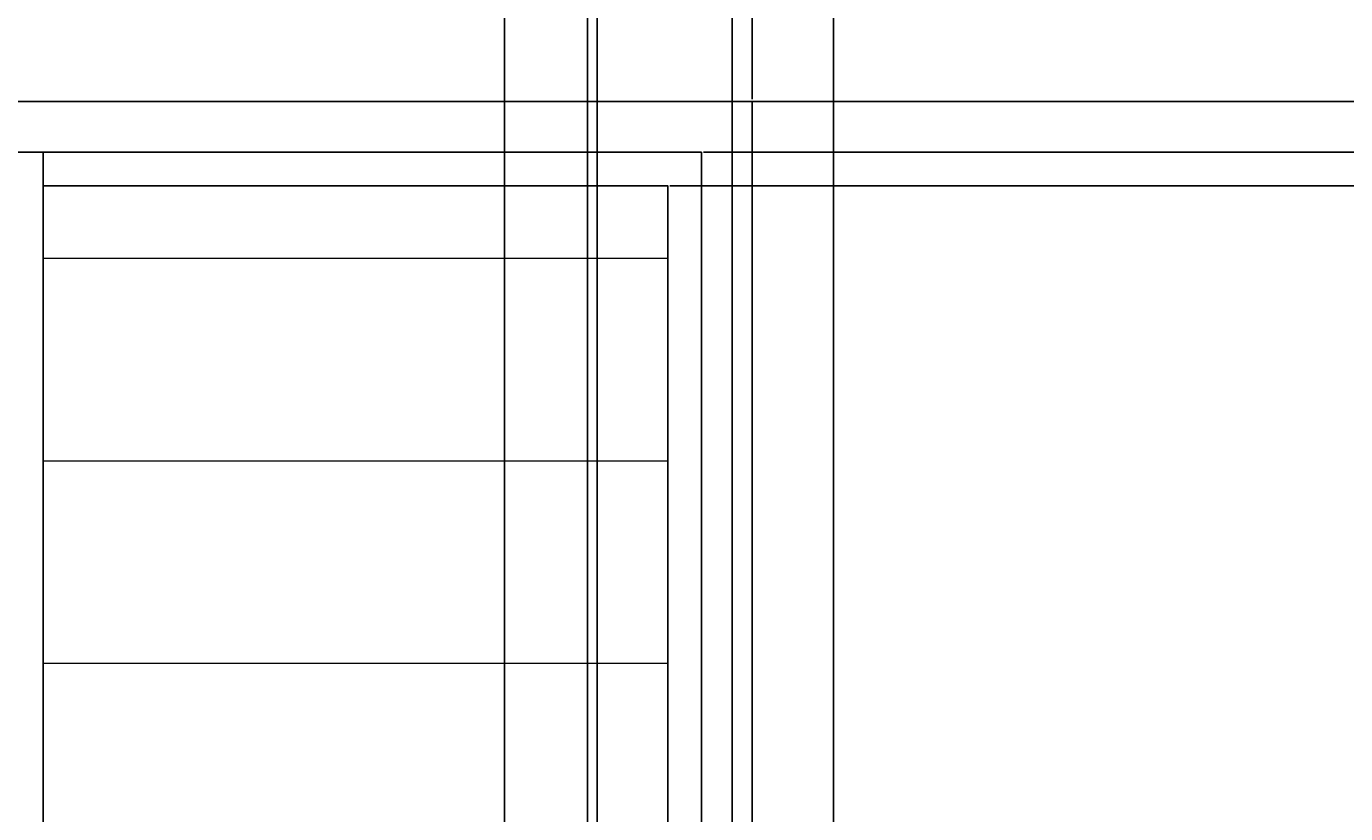
# Model space of a CAD drawing. Units: inches. Extents: x -6 to 289, y -8 to 323.
# Tile 61 of 107: x 147 to 186, y 206 to 229. Entities that reach past the tile are written whole.
import ezdxf

# ---------------------------------------------------------------- set-up
doc = ezdxf.new("R2010")
doc.units = ezdxf.units.IN
doc.header["$MEASUREMENT"] = 0
for name, color, linetype, lineweight in [('A-ANNO-DIMS', 2, 'Continuous', 18), ('A-ELEV-PATT', 8, 'Continuous', 13), ('A-GLAZ', 4, 'Continuous', 25)]:
    doc.layers.add(name, color=color, linetype=linetype, lineweight=lineweight)
doc.styles.get("Standard").update_dxf_attribs({"font": 'arial.ttf'})
doc.dimstyles.get("Standard").update_dxf_attribs({"dimtxt": 0.18, "dimasz": 0.18, "dimexe": 0.18, "dimexo": 0.0625, "dimgap": 0.09, "dimtad": 0, "dimtih": 1, "dimtoh": 1, "dimdec": 4, "dimzin": 0, "dimdsep": 46, "dimtxsty": 'Standard', "dimcen": 0.09, "dimadec": 0, "dimazin": 0, "dimtfac": 1, "dimtdec": 4, "dimtofl": 0, "dimtmove": 0, "dimatfit": 3, "dimfxl": 1, "dimtolj": 1, "dimtzin": 0, "dimarcsym": 0})

# ---------------------------------------------------------------- blocks, each defined once
blk = doc.blocks.new('*U4')
for p, q in [((1.5, 46.5), (21, 46.5)), ((21, 1.5), (21, 46.5)), ((21, 46.5), (40.5, 46.5)), ((40.5, 46.5), (40.5, 1.5))]:
    blk.add_line(p, q)
blk.add_lwpolyline([(0, 0), (0, 48), (42, 48), (42, 0)], close=True)
blk.add_lwpolyline([(21, 45.5), (39.5, 45.5), (39.5, 2.5), (21, 2.5)])
blk = doc.blocks.new('*D11')
at = {"layer": 'A-ANNO-DIMS', "color": 0, "lineweight": -2, "transparency": 16777216}
for p, q in [((126.883, 226.717), (126.883, 322.969)), ((168.883, 226.717), (168.883, 322.969)), ((127.063, 322.789), (147.662, 322.789)), ((168.703, 322.789), (148.105, 322.789))]:
    blk.add_line(p, q, dxfattribs=at)
at = {"layer": 'A-ANNO-DIMS', "color": 0, "transparency": 16777216}
for points in [[(127.063, 322.819), (127.063, 322.759), (126.883, 322.789)], [(168.703, 322.819), (168.703, 322.759), (168.883, 322.789)]]:
    blk.add_solid(points, dxfattribs=at)
at = {"layer": 'Defpoints', "color": 0, "transparency": 16777216}
for p in [(168.883, 322.789), (126.883, 226.654), (168.883, 226.654)]:
    blk.add_point(p, dxfattribs=at)
at = {"layer": 'A-ANNO-DIMS', "color": 0, "transparency": 16777216, "insert": (147.883, 322.789), "char_height": 0.18, "attachment_point": 5}
blk.add_mtext('\\A1;42', dxfattribs=at)
blk = doc.blocks.new('*D12')
at = {"layer": 'A-ANNO-DIMS', "color": 0, "lineweight": -2, "transparency": 16777216}
for p, q in [((168.883, 226.717), (168.883, 322.969)), ((188.292, 226.951), (188.292, 322.969)), ((169.063, 322.789), (178.22, 322.789)), ((188.112, 322.789), (178.955, 322.789))]:
    blk.add_line(p, q, dxfattribs=at)
at = {"layer": 'A-ANNO-DIMS', "color": 0, "transparency": 16777216}
for points in [[(169.063, 322.819), (169.063, 322.759), (168.883, 322.789)], [(188.112, 322.819), (188.112, 322.759), (188.292, 322.789)]]:
    blk.add_solid(points, dxfattribs=at)
at = {"layer": 'Defpoints', "color": 0, "transparency": 16777216}
for p in [(188.292, 322.789), (188.292, 226.889), (168.883, 226.654)]:
    blk.add_point(p, dxfattribs=at)
at = {"layer": 'A-ANNO-DIMS', "color": 0, "transparency": 16777216, "insert": (178.588, 322.789), "char_height": 0.18, "attachment_point": 5}
blk.add_mtext('\\A1;19.41', dxfattribs=at)
blk = doc.blocks.new('*D25')
at = {"layer": 'A-ANNO-DIMS', "color": 0, "lineweight": -2, "transparency": 16777216}
for p, q in [((126.946, 226.654), (288.653, 226.654)), ((288.473, 226.474), (288.473, 202.836)), ((288.473, 178.834), (288.473, 202.472)), ((126.946, 178.654), (288.653, 178.654))]:
    blk.add_line(p, q, dxfattribs=at)
at = {"layer": 'A-ANNO-DIMS', "color": 0, "transparency": 16777216}
for points in [[(288.443, 226.474), (288.503, 226.474), (288.473, 226.654)], [(288.443, 178.834), (288.503, 178.834), (288.473, 178.654)]]:
    blk.add_solid(points, dxfattribs=at)
at = {"layer": 'Defpoints', "color": 0, "transparency": 16777216}
for p in [(126.883, 226.654), (288.473, 226.654), (126.883, 178.654)]:
    blk.add_point(p, dxfattribs=at)
at = {"layer": 'A-ANNO-DIMS', "color": 0, "transparency": 16777216, "insert": (288.473, 202.654), "char_height": 0.18, "attachment_point": 5}
blk.add_mtext('\\A1;48', dxfattribs=at)
blk = doc.blocks.new('*D26')
at = {"layer": 'A-ANNO-DIMS', "color": 0, "lineweight": -2, "transparency": 16777216}
for p, q in [((247.226, 247.289), (288.653, 247.289)), ((288.473, 247.109), (288.473, 237.153)), ((288.473, 226.834), (288.473, 236.789)), ((126.946, 226.654), (288.653, 226.654))]:
    blk.add_line(p, q, dxfattribs=at)
at = {"layer": 'A-ANNO-DIMS', "color": 0, "transparency": 16777216}
for points in [[(288.443, 247.109), (288.503, 247.109), (288.473, 247.289)], [(288.443, 226.834), (288.503, 226.834), (288.473, 226.654)]]:
    blk.add_solid(points, dxfattribs=at)
at = {"layer": 'Defpoints', "color": 0, "transparency": 16777216}
for p in [(247.164, 247.289), (288.473, 247.289), (126.883, 226.654)]:
    blk.add_point(p, dxfattribs=at)
at = {"layer": 'A-ANNO-DIMS', "color": 0, "transparency": 16777216, "insert": (288.473, 236.971), "char_height": 0.18, "attachment_point": 5}
blk.add_mtext('\\A1;20.635', dxfattribs=at)
blk = doc.blocks.new('*D37')
at = {"layer": 'A-ANNO-DIMS', "color": 0, "lineweight": -2, "transparency": 16777216}
for p, q in [((166.446, 224.154), (288.653, 224.154)), ((288.473, 223.974), (288.473, 202.836)), ((288.473, 181.334), (288.473, 202.472)), ((166.446, 181.154), (288.653, 181.154))]:
    blk.add_line(p, q, dxfattribs=at)
at = {"layer": 'A-ANNO-DIMS', "color": 0, "transparency": 16777216}
for points in [[(288.443, 223.974), (288.503, 223.974), (288.473, 224.154)], [(288.443, 181.334), (288.503, 181.334), (288.473, 181.154)]]:
    blk.add_solid(points, dxfattribs=at)
at = {"layer": 'Defpoints', "color": 0, "transparency": 16777216}
for p in [(166.383, 224.154), (288.473, 224.154), (166.383, 181.154)]:
    blk.add_point(p, dxfattribs=at)
at = {"layer": 'A-ANNO-DIMS', "color": 0, "transparency": 16777216, "insert": (288.473, 202.654), "char_height": 0.18, "attachment_point": 5}
blk.add_mtext('\\A1;43', dxfattribs=at)
blk = doc.blocks.new('*D38')
at = {"layer": 'A-ANNO-DIMS', "color": 0, "lineweight": -2, "transparency": 16777216}
for p, q in [((167.446, 225.154), (288.653, 225.154)), ((288.473, 224.974), (288.473, 224.834)), ((288.473, 224.334), (288.473, 224.474)), ((166.446, 224.154), (288.653, 224.154))]:
    blk.add_line(p, q, dxfattribs=at)
at = {"layer": 'A-ANNO-DIMS', "color": 0, "transparency": 16777216}
for points in [[(288.443, 224.974), (288.503, 224.974), (288.473, 225.154)], [(288.443, 224.334), (288.503, 224.334), (288.473, 224.154)]]:
    blk.add_solid(points, dxfattribs=at)
at = {"layer": 'Defpoints', "color": 0, "transparency": 16777216}
for p in [(167.383, 225.154), (288.473, 225.154), (166.383, 224.154)]:
    blk.add_point(p, dxfattribs=at)
at = {"layer": 'A-ANNO-DIMS', "color": 0, "transparency": 16777216, "insert": (288.473, 224.654), "char_height": 0.18, "attachment_point": 5}
blk.add_mtext('\\A1;1', dxfattribs=at)
blk = doc.blocks.new('*D39')
at = {"layer": 'A-ANNO-DIMS', "color": 0, "lineweight": -2, "transparency": 16777216}
for p, q in [((168.946, 226.654), (288.653, 226.654)), ((288.473, 226.474), (288.473, 226.086)), ((288.473, 225.334), (288.473, 225.722)), ((167.446, 225.154), (288.653, 225.154))]:
    blk.add_line(p, q, dxfattribs=at)
at = {"layer": 'A-ANNO-DIMS', "color": 0, "transparency": 16777216}
for points in [[(288.443, 226.474), (288.503, 226.474), (288.473, 226.654)], [(288.443, 225.334), (288.503, 225.334), (288.473, 225.154)]]:
    blk.add_solid(points, dxfattribs=at)
at = {"layer": 'Defpoints', "color": 0, "transparency": 16777216}
for p in [(168.883, 226.654), (288.473, 226.654), (167.383, 225.154)]:
    blk.add_point(p, dxfattribs=at)
at = {"layer": 'A-ANNO-DIMS', "color": 0, "transparency": 16777216, "insert": (288.473, 225.904), "char_height": 0.18, "attachment_point": 5}
blk.add_mtext('\\A1;1.5', dxfattribs=at)
blk = doc.blocks.new('*D76')
at = {"layer": 'A-ANNO-DIMS', "color": 0, "lineweight": -2, "transparency": 16777216}
for p, q in [((142.296, 51.148), (142.296, 322.969)), ((164.296, 51.148), (164.296, 322.969)), ((142.476, 322.789), (153.076, 322.789)), ((164.116, 322.789), (153.516, 322.789))]:
    blk.add_line(p, q, dxfattribs=at)
at = {"layer": 'A-ANNO-DIMS', "color": 0, "transparency": 16777216}
for points in [[(142.476, 322.819), (142.476, 322.759), (142.296, 322.789)], [(164.116, 322.819), (164.116, 322.759), (164.296, 322.789)]]:
    blk.add_solid(points, dxfattribs=at)
at = {"layer": 'Defpoints', "color": 0, "transparency": 16777216}
for p in [(164.296, 322.789), (142.296, 51.085), (164.296, 51.085)]:
    blk.add_point(p, dxfattribs=at)
at = {"layer": 'A-ANNO-DIMS', "color": 0, "transparency": 16777216, "insert": (153.296, 322.789), "char_height": 0.18, "attachment_point": 5}
blk.add_mtext('\\A1;22', dxfattribs=at)
blk = doc.blocks.new('*D77')
at = {"layer": 'A-ANNO-DIMS', "color": 0, "lineweight": -2, "transparency": 16777216}
for p, q in [((164.296, 51.148), (164.296, 322.969)), ((168.296, 51.148), (168.296, 322.969)), ((164.476, 322.789), (166.144, 322.789)), ((168.116, 322.789), (166.448, 322.789))]:
    blk.add_line(p, q, dxfattribs=at)
at = {"layer": 'A-ANNO-DIMS', "color": 0, "transparency": 16777216}
for points in [[(164.476, 322.819), (164.476, 322.759), (164.296, 322.789)], [(168.116, 322.819), (168.116, 322.759), (168.296, 322.789)]]:
    blk.add_solid(points, dxfattribs=at)
at = {"layer": 'Defpoints', "color": 0, "transparency": 16777216}
for p in [(168.296, 322.789), (164.296, 51.085), (168.296, 51.085)]:
    blk.add_point(p, dxfattribs=at)
at = {"layer": 'A-ANNO-DIMS', "color": 0, "transparency": 16777216, "insert": (166.296, 322.789), "char_height": 0.18, "attachment_point": 5}
blk.add_mtext('\\A1;4', dxfattribs=at)
blk = doc.blocks.new('*D78')
at = {"layer": 'A-ANNO-DIMS', "color": 0, "lineweight": -2, "transparency": 16777216}
for p, q in [((168.296, 51.148), (168.296, 322.969)), ((171.296, 51.148), (171.296, 322.969)), ((168.476, 322.789), (169.647, 322.789)), ((171.116, 322.789), (169.945, 322.789))]:
    blk.add_line(p, q, dxfattribs=at)
at = {"layer": 'A-ANNO-DIMS', "color": 0, "transparency": 16777216}
for points in [[(168.476, 322.819), (168.476, 322.759), (168.296, 322.789)], [(171.116, 322.819), (171.116, 322.759), (171.296, 322.789)]]:
    blk.add_solid(points, dxfattribs=at)
at = {"layer": 'Defpoints', "color": 0, "transparency": 16777216}
for p in [(171.296, 322.789), (168.296, 51.085), (171.296, 51.085)]:
    blk.add_point(p, dxfattribs=at)
at = {"layer": 'A-ANNO-DIMS', "color": 0, "transparency": 16777216, "insert": (169.796, 322.789), "char_height": 0.18, "attachment_point": 5}
blk.add_mtext('\\A1;3', dxfattribs=at)
blk = doc.blocks.new('*D79')
at = {"layer": 'A-ANNO-DIMS', "color": 0, "lineweight": -2, "transparency": 16777216}
for p, q in [((171.296, 118.033), (171.296, 322.969)), ((188.292, 116.842), (188.292, 322.969)), ((171.476, 322.789), (179.339, 322.789)), ((188.112, 322.789), (180.249, 322.789))]:
    blk.add_line(p, q, dxfattribs=at)
at = {"layer": 'A-ANNO-DIMS', "color": 0, "transparency": 16777216}
for points in [[(171.476, 322.819), (171.476, 322.759), (171.296, 322.789)], [(188.112, 322.819), (188.112, 322.759), (188.292, 322.789)]]:
    blk.add_solid(points, dxfattribs=at)
at = {"layer": 'Defpoints', "color": 0, "transparency": 16777216}
for p in [(188.292, 322.789), (171.296, 117.971), (188.292, 116.779)]:
    blk.add_point(p, dxfattribs=at)
at = {"layer": 'A-ANNO-DIMS', "color": 0, "transparency": 16777216, "insert": (179.794, 322.789), "char_height": 0.18, "attachment_point": 5}
blk.add_mtext('\\A1;16.996', dxfattribs=at)
blk = doc.blocks.new('*D94')
at = {"layer": 'A-ANNO-DIMS', "color": 0, "lineweight": -2, "transparency": 16777216}
for p, q in [((118.164, 159.411), (118.164, 322.969)), ((161.552, 159.411), (161.552, 322.969)), ((118.344, 322.789), (139.46, 322.789)), ((161.372, 322.789), (140.256, 322.789))]:
    blk.add_line(p, q, dxfattribs=at)
at = {"layer": 'A-ANNO-DIMS', "color": 0, "transparency": 16777216}
for points in [[(118.344, 322.819), (118.344, 322.759), (118.164, 322.789)], [(161.372, 322.819), (161.372, 322.759), (161.552, 322.789)]]:
    blk.add_solid(points, dxfattribs=at)
at = {"layer": 'Defpoints', "color": 0, "transparency": 16777216}
for p in [(161.552, 322.789), (118.164, 159.348), (161.552, 159.348)]:
    blk.add_point(p, dxfattribs=at)
at = {"layer": 'A-ANNO-DIMS', "color": 0, "transparency": 16777216, "insert": (139.858, 322.789), "char_height": 0.18, "attachment_point": 5}
blk.add_mtext('\\A1;43.39', dxfattribs=at)
blk = doc.blocks.new('*D95')
at = {"layer": 'A-ANNO-DIMS', "color": 0, "lineweight": -2, "transparency": 16777216}
for p, q in [((161.552, 159.411), (161.552, 322.969)), ((164.004, 159.411), (164.004, 322.969)), ((161.732, 322.789), (162.452, 322.789)), ((163.824, 322.789), (163.104, 322.789))]:
    blk.add_line(p, q, dxfattribs=at)
at = {"layer": 'A-ANNO-DIMS', "color": 0, "transparency": 16777216}
for points in [[(161.732, 322.819), (161.732, 322.759), (161.552, 322.789)], [(163.824, 322.819), (163.824, 322.759), (164.004, 322.789)]]:
    blk.add_solid(points, dxfattribs=at)
at = {"layer": 'Defpoints', "color": 0, "transparency": 16777216}
for p in [(164.004, 322.789), (161.552, 159.348), (164.004, 159.348)]:
    blk.add_point(p, dxfattribs=at)
at = {"layer": 'A-ANNO-DIMS', "color": 0, "transparency": 16777216, "insert": (162.778, 322.789), "char_height": 0.18, "attachment_point": 5}
blk.add_mtext('\\A1;2.45', dxfattribs=at)
blk = doc.blocks.new('*D96')
at = {"layer": 'A-ANNO-DIMS', "color": 0, "lineweight": -2, "transparency": 16777216}
for p, q in [((164.004, 159.411), (164.004, 322.969)), ((200.616, 159.411), (200.616, 322.969)), ((164.184, 322.789), (181.934, 322.789)), ((200.436, 322.789), (182.686, 322.789))]:
    blk.add_line(p, q, dxfattribs=at)
at = {"layer": 'A-ANNO-DIMS', "color": 0, "transparency": 16777216}
for points in [[(164.184, 322.819), (164.184, 322.759), (164.004, 322.789)], [(200.436, 322.819), (200.436, 322.759), (200.616, 322.789)]]:
    blk.add_solid(points, dxfattribs=at)
at = {"layer": 'Defpoints', "color": 0, "transparency": 16777216}
for p in [(200.616, 322.789), (164.004, 159.348), (200.616, 159.348)]:
    blk.add_point(p, dxfattribs=at)
at = {"layer": 'A-ANNO-DIMS', "color": 0, "transparency": 16777216, "insert": (182.31, 322.789), "char_height": 0.18, "attachment_point": 5}
blk.add_mtext('\\A1;36.61', dxfattribs=at)

msp = doc.modelspace()

# ---------------------------------------------------------------- hatches: boundary and pattern name
at = {"layer": 'A-ELEV-PATT'}
h = msp.add_hatch(dxfattribs=at)
h.set_pattern_fill('_USER', color=256, scale=6, pattern_type=0)
h.set_pattern_definition([(0, (0, 0), (0, 6), [])])
h.paths.add_polyline_path([(184.1244, 48.0851), (124.008, 48.0851), (124.008, 10.2888), (184.1244, 10.2888)])
h.paths.add_polyline_path([(244.2408, 48.0851), (186.3604, 48.0851), (186.3604, 10.2888), (244.2408, 10.2888)])
h.paths.add_polyline_path([(208.2918, 114.2795), (190.7918, 114.2795), (190.7918, 71.2795), (208.2918, 71.2795)])
h.paths.add_polyline_path([(227.7918, 114.2795), (209.2918, 114.2795), (209.2918, 71.2795), (227.7918, 71.2795)])
h.paths.add_polyline_path([(211.2918, 224.3887), (190.7918, 224.3887), (190.7918, 162.3484), (211.2918, 162.3484)])
h.paths.add_polyline_path([(233.7918, 224.3887), (212.2918, 224.3887), (212.2918, 162.3484), (233.7918, 162.3484)])
h.paths.add_polyline_path([(166.3835, 224.154), (147.8835, 224.154), (147.8835, 181.154), (166.3835, 181.154)])
h.paths.add_polyline_path([(146.8835, 224.154), (129.3835, 224.154), (129.3835, 181.154), (146.8835, 181.154)])

# ---------------------------------------------------------------- block references
at = {"layer": 'A-GLAZ'}
msp.add_blockref('*U4', (126.8835, 178.654), dxfattribs=at)

# ---------------------------------------------------------------- dimensions: what is measured, and where the dimension line sits
at = {"layer": 'A-ANNO-DIMS'}
for base, p1, p2, override, picture, middle in [((161.5522, 322.7888), (118.1638, 159.3484), (161.5522, 159.3484), {"dimdec": 2, "dimlfac": 1, "dimrnd": 0, "dimzin": 0, "dimdsep": 46, "dimlunit": 2}, '*D94', (139.858, 322.7888)), ((168.8835, 322.7888), (126.8835, 226.654), (168.8835, 226.654), {"dimdec": 0, "dimlfac": 1, "dimrnd": 0, "dimzin": 0, "dimdsep": 46, "dimlunit": 2}, '*D11', (147.8835, 322.7888)), ((164.296, 322.7888), (142.296, 51.0851), (164.296, 51.0851), {"dimdec": 0, "dimlfac": 1, "dimrnd": 0, "dimzin": 0, "dimdsep": 46, "dimlunit": 2}, '*D76', (153.296, 322.7888)), ((164.0039, 322.7888), (161.5522, 159.3484), (164.0039, 159.3484), {"dimdec": 2, "dimlfac": 1, "dimrnd": 0, "dimzin": 0, "dimdsep": 46, "dimlunit": 2}, '*D95', (162.7781, 322.7888)), ((200.6162, 322.7888), (164.0039, 159.3484), (200.6162, 159.3484), {"dimdec": 2, "dimlfac": 1, "dimrnd": 0, "dimzin": 0, "dimdsep": 46, "dimlunit": 2}, '*D96', (182.3101, 322.7888)), ((168.296, 322.7888), (164.296, 51.0851), (168.296, 51.0851), {"dimdec": 0, "dimlfac": 1, "dimrnd": 0, "dimzin": 0, "dimdsep": 46, "dimlunit": 2}, '*D77', (166.296, 322.7888)), ((171.296, 322.7888), (168.296, 51.0851), (171.296, 51.0851), {"dimdec": 0, "dimlfac": 1, "dimrnd": 0, "dimzin": 0, "dimdsep": 46, "dimlunit": 2}, '*D78', (169.796, 322.7888)), ((188.2918, 322.7888), (168.8835, 226.654), (188.2918, 226.8887), {"dimdec": 2, "dimlfac": 1, "dimrnd": 0, "dimzin": 0, "dimdsep": 46, "dimlunit": 2}, '*D12', (178.5876, 322.7888)), ((188.2918, 322.7888), (171.296, 117.9706), (188.2918, 116.7795), {"dimdec": 3, "dimlfac": 1, "dimrnd": 0, "dimzin": 0, "dimdsep": 46, "dimlunit": 2}, '*D79', (179.7939, 322.7888))]:
    dim = msp.add_linear_dim(base=base, p1=p1, p2=p2, dimstyle='Standard', override=override, dxfattribs=at)
    dim.commit()
    dim.dimension.update_dxf_attribs({"geometry": picture, "text_midpoint": middle})
for base, p1, p2, override, picture, middle in [((288.4733, 247.2888), (126.8835, 226.654), (247.1638, 247.2888), {"dimdec": 3, "dimlfac": 1, "dimrnd": 0, "dimzin": 0, "dimdsep": 46, "dimlunit": 2}, '*D26', (288.4733, 236.9714)), ((288.4733, 226.654), (126.8835, 178.654), (126.8835, 226.654), {"dimdec": 0, "dimlfac": 1, "dimrnd": 0, "dimzin": 0, "dimdsep": 46, "dimlunit": 2}, '*D25', (288.4733, 202.654)), ((288.4733, 226.654), (167.3835, 225.154), (168.8835, 226.654), {"dimdec": 1, "dimlfac": 1, "dimrnd": 0, "dimzin": 0, "dimdsep": 46, "dimlunit": 2}, '*D39', (288.4733, 225.904)), ((288.4733, 225.154), (166.3835, 224.154), (167.3835, 225.154), {"dimdec": 0, "dimlfac": 1, "dimrnd": 0, "dimzin": 0, "dimdsep": 46, "dimlunit": 2}, '*D38', (288.4733, 224.654)), ((288.4733, 224.154), (166.3835, 181.154), (166.3835, 224.154), {"dimdec": 0, "dimlfac": 1, "dimrnd": 0, "dimzin": 0, "dimdsep": 46, "dimlunit": 2}, '*D37', (288.4733, 202.654))]:
    dim = msp.add_linear_dim(base=base, p1=p1, p2=p2, angle=90, dimstyle='Standard', override=override, dxfattribs=at)
    dim.commit()
    dim.dimension.update_dxf_attribs({"geometry": picture, "text_midpoint": middle})

doc.saveas('drawing.dxf')
